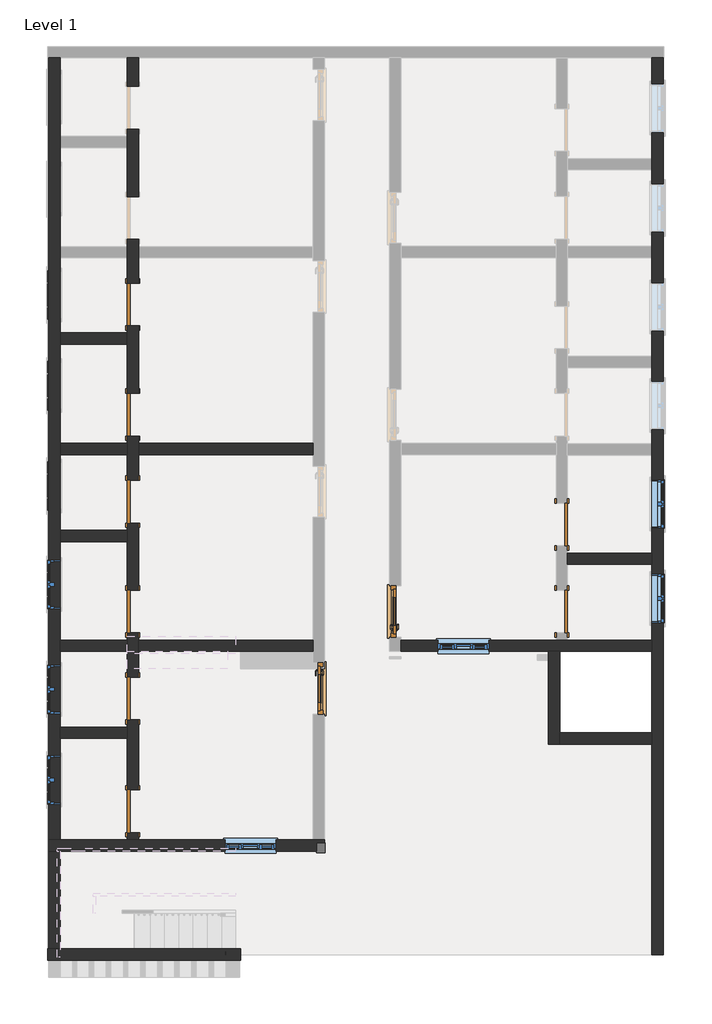
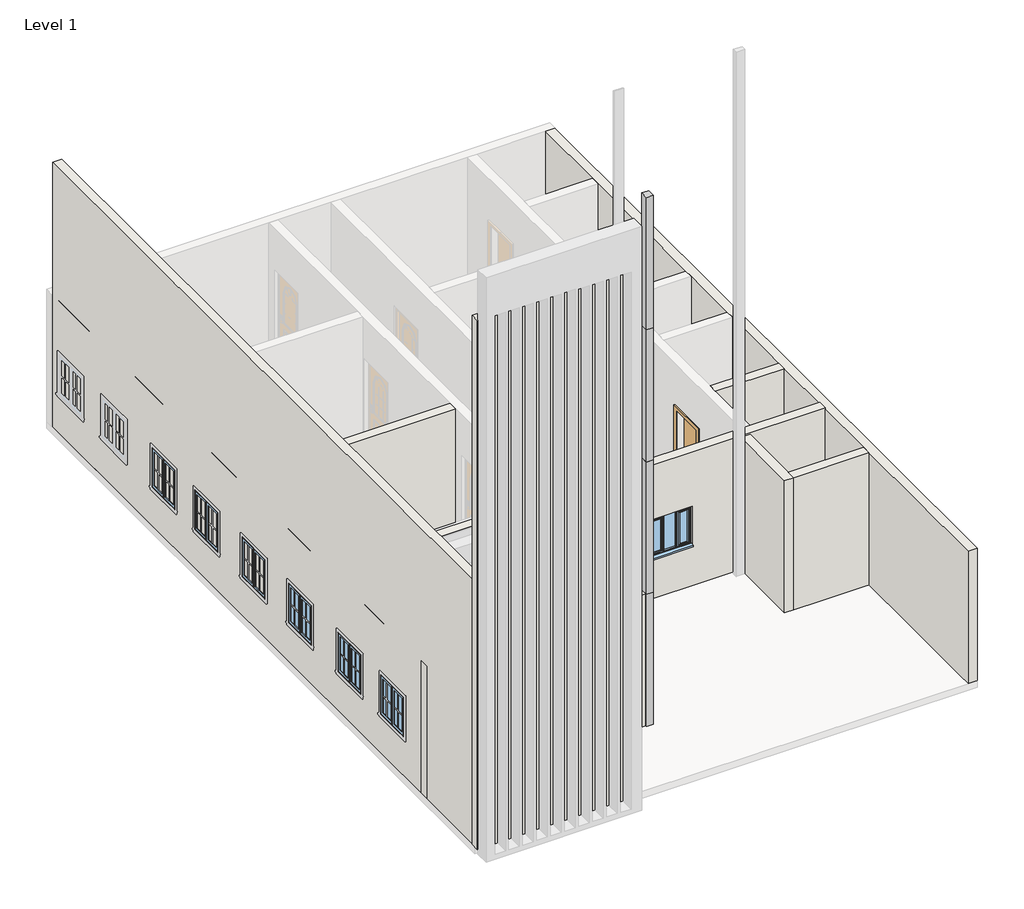
# One storey, part 1 of 4: 17 walls, 10 doors, 10 windows, 1 proxy.
"""IFC4 building model written with IfcOpenShell, lengths in millimetres."""

from ifc_helpers import new_model, si_unit, frame, origin, origin_with_axes, place, context, project, spatial, polyline, outline, extrude, faceted_brep, transform, mapped, element, save
from components import doors_extsgl_w_glazing_bars_arched_910x2110mm_1ab485ba, door_fadea3f2, door_53b1b562, window_c29befe5, windows_tpl_plain_910x910mm_84e79c20

model = new_model("IFC4")

# Units and contexts
model_context = context("Model", 3, world=origin())
ifc_project = project(units=[si_unit("LENGTHUNIT", "METRE", prefix="MILLI")], contexts=[model_context])

# Site, building, storey
site = spatial("IfcSite", under=ifc_project)
building = spatial("IfcBuilding", under=site)
storey = spatial("IfcBuildingStorey", under=building, Name="Level 1", Elevation=0.0)

# Proxy
placement = place(None, origin())
element("IfcBuildingElementProxy", 1, Name="Reveal", ObjectType="Reveal", at=placement, inside=storey, context=model_context, shape_type="SweptSolid", body=[
    extrude(outline(polyline([(-1673.2108866, -6357.2400272), (-1673.2108866, -6174.3600272), (-1520.8108866, -6174.3600272), (-1520.8108866, -6357.2400272), (-1673.2108866, -6357.2400272)])), frame((0.0, 0.0, 9144.0), z_axis=(0.0, 0.0, 1.0), x_axis=(1.0, 0.0, 0.0)), (0.0, 0.0, 1.0), 3048.0),
    extrude(outline(polyline([(-1673.2108866, -6357.2400272), (-1673.2108866, -6174.3600272), (-1520.8108866, -6174.3600272), (-1520.8108866, -6357.2400272), (-1673.2108866, -6357.2400272)])), frame((0.0, 0.0, 6096.0), z_axis=(0.0, 0.0, 1.0), x_axis=(1.0, 0.0, 0.0)), (0.0, 0.0, 1.0), 3048.0),
    extrude(outline(polyline([(-1673.2108866, -6357.2400272), (-1673.2108866, -6174.3600272), (-1520.8108866, -6174.3600272), (-1520.8108866, -6357.2400272), (-1673.2108866, -6357.2400272)])), frame((0.0, 0.0, 3048.0), z_axis=(0.0, 0.0, 1.0), x_axis=(1.0, 0.0, 0.0)), (0.0, 0.0, 1.0), 3048.0),
    extrude(outline(polyline([(-1673.2108866, -6357.2400272), (-1673.2108866, -6174.3600272), (-1520.8108866, -6174.3600272), (-1520.8108866, -6357.2400272), (-1673.2108866, -6357.2400272)])), origin_with_axes(), (0.0, 0.0, 1.0), 3048.0),
])

# Doors
doors_extsgl_w_glazing_bars_arched_910x2110mm_shape = doors_extsgl_w_glazing_bars_arched_910x2110mm_1ab485ba(model_context)
element("IfcDoor", 2, ObjectType="Doors_ExtSgl_w-Glazing_Bars_Arched : 910x2110mm", at=placement, inside=storey, context=model_context, shape_type="MappedRepresentation", body=[
    mapped(doors_extsgl_w_glazing_bars_arched_910x2110mm_shape, transform((-1635.1108866, -3431.1600272, 0.0), x_axis=(0.0, -1.0, 0.0), y_axis=(1.0, 0.0, 0.0), z_axis=(0.0, 0.0, 1.0))),
])
element("IfcDoor", 3, ObjectType="Doors_ExtSgl_w-Glazing_Bars_Arched : 910x2110mm", at=placement, inside=storey, context=model_context, shape_type="MappedRepresentation", body=[
    mapped(doors_extsgl_w_glazing_bars_arched_910x2110mm_shape, transform((-276.2108866, -2059.5600272, 0.0), x_axis=(0.0, 1.0, 0.0), y_axis=(-1.0, 0.0, 0.0), z_axis=(0.0, 0.0, 1.0))),
])
door_shape = door_fadea3f2(model_context)
element("IfcDoor", 4, ObjectType="Single-Flush : 30\" x 80\"", at=placement, inside=storey, context=model_context, shape_type="MappedRepresentation", body=[
    mapped(door_shape, transform((2695.5891134, -510.1600272, 0.0), x_axis=(0.0, -1.0, 0.0), y_axis=(1.0, 0.0, 0.0), z_axis=(0.0, 0.0, 1.0))),
])
element("IfcDoor", 5, ObjectType="Single-Flush : 30\" x 80\"", at=placement, inside=storey, context=model_context, shape_type="MappedRepresentation", body=[
    mapped(door_shape, transform((2695.5891134, -2059.5600272, 0.0), x_axis=(0.0, -1.0, 0.0), y_axis=(1.0, 0.0, 0.0), z_axis=(0.0, 0.0, 1.0))),
])
door_2_shape = door_53b1b562(model_context)
element("IfcDoor", 6, ObjectType="Single-Flush : 30\" x 80\"", at=placement, inside=storey, context=model_context, shape_type="MappedRepresentation", body=[
    mapped(door_2_shape, transform((-4949.8108866, 3407.538843, 0.0), x_axis=(0.0, -1.0, 0.0), y_axis=(1.0, 0.0, 0.0), z_axis=(0.0, 0.0, 1.0))),
])
element("IfcDoor", 7, ObjectType="Single-Flush : 30\" x 80\"", at=placement, inside=storey, context=model_context, shape_type="MappedRepresentation", body=[
    mapped(door_2_shape, transform((-4949.8108866, 1445.6399728, 0.0), x_axis=(0.0, -1.0, 0.0), y_axis=(1.0, 0.0, 0.0), z_axis=(0.0, 0.0, 1.0))),
])
element("IfcDoor", 8, ObjectType="Single-Flush : 30\" x 80\"", at=placement, inside=storey, context=model_context, shape_type="MappedRepresentation", body=[
    mapped(door_2_shape, transform((-4949.8108866, -103.7600272, 0.0), x_axis=(0.0, -1.0, 0.0), y_axis=(1.0, 0.0, 0.0), z_axis=(0.0, 0.0, 1.0))),
])
element("IfcDoor", 9, ObjectType="Single-Flush : 30\" x 80\"", at=placement, inside=storey, context=model_context, shape_type="MappedRepresentation", body=[
    mapped(door_2_shape, transform((-4949.8108866, -2059.5600272, 0.0), x_axis=(0.0, -1.0, 0.0), y_axis=(1.0, 0.0, 0.0), z_axis=(0.0, 0.0, 1.0))),
])
element("IfcDoor", 10, ObjectType="Single-Flush : 30\" x 80\"", at=placement, inside=storey, context=model_context, shape_type="MappedRepresentation", body=[
    mapped(door_2_shape, transform((-4949.8108866, -3608.9600272, 0.0), x_axis=(0.0, -1.0, 0.0), y_axis=(1.0, 0.0, 0.0), z_axis=(0.0, 0.0, 1.0))),
])
element("IfcDoor", 11, ObjectType="Single-Flush : 30\" x 80\"", at=placement, inside=storey, context=model_context, shape_type="MappedRepresentation", body=[
    mapped(door_2_shape, transform((-4949.8108866, -5615.5600272, 0.0), x_axis=(0.0, -1.0, 0.0), y_axis=(1.0, 0.0, 0.0), z_axis=(0.0, 0.0, 1.0))),
])

# Walls
element("IfcWall", 12, ObjectType="4.5\" p", at=placement, inside=storey, context=model_context, shape_type="Brep", body=[
    faceted_brep([(-5051.4108866, -5996.5600272, 2032.0), (-5051.4108866, -5996.5600272, 0.0), (-5051.4108866, -6123.5600272, 0.0), (-5051.4108866, -6123.5600272, 3048.0), (-5051.4108866, -4320.1600272, 3048.0), (-5051.4108866, -4116.9600272, 3048.0), (-5051.4108866, -2770.7600272, 3048.0), (-5051.4108866, -2567.5600272, 3048.0), (-5051.4108866, -814.9600272, 3048.0), (-5051.4108866, -611.7600272, 3048.0), (-5051.4108866, 734.4399728, 3048.0), (-5051.4108866, 937.6399728, 3048.0), (-5051.4108866, 2696.338843, 3048.0), (-5051.4108866, 2899.538843, 3048.0), (-5051.4108866, 4235.1935874, 3048.0), (-5051.4108866, 4438.3935874, 3048.0), (-5051.4108866, 6195.4399728, 3048.0), (-5051.4108866, 6398.6399728, 3048.0), (-5051.4108866, 7795.6399728, 3048.0), (-5051.4108866, 7795.6399728, 0.0), (-5051.4108866, 7287.6399728, 0.0), (-5051.4108866, 7287.6399728, 2032.0), (-5051.4108866, 6525.6399728, 2032.0), (-5051.4108866, 6525.6399728, 0.0), (-5051.4108866, 6398.6399728, 0.0), (-5051.4108866, 6195.4399728, 0.0), (-5051.4108866, 5327.3935874, 0.0), (-5051.4108866, 5327.3935874, 2032.0), (-5051.4108866, 4565.3935874, 2032.0), (-5051.4108866, 4565.3935874, 0.0), (-5051.4108866, 4438.3935874, 0.0), (-5051.4108866, 4235.1935874, 0.0), (-5051.4108866, 3788.538843, 0.0), (-5051.4108866, 3788.538843, 2032.0), (-5051.4108866, 3026.538843, 2032.0), (-5051.4108866, 3026.538843, 0.0), (-5051.4108866, 2899.538843, 0.0), (-5051.4108866, 2696.338843, 0.0), (-5051.4108866, 1826.6399728, 0.0), (-5051.4108866, 1826.6399728, 2032.0), (-5051.4108866, 1064.6399728, 2032.0), (-5051.4108866, 1064.6399728, 0.0), (-5051.4108866, 937.6399728, 0.0), (-5051.4108866, 734.4399728, 0.0), (-5051.4108866, 277.2399728, 0.0), (-5051.4108866, 277.2399728, 2032.0), (-5051.4108866, -484.7600272, 2032.0), (-5051.4108866, -484.7600272, 0.0), (-5051.4108866, -611.7600272, 0.0), (-5051.4108866, -814.9600272, 0.0), (-5051.4108866, -1678.5600272, 0.0), (-5051.4108866, -1678.5600272, 2032.0), (-5051.4108866, -2440.5600272, 2032.0), (-5051.4108866, -2440.5600272, 0.0), (-5051.4108866, -2567.5600272, 0.0), (-5051.4108866, -2770.7600272, 0.0), (-5051.4108866, -3227.9600272, 0.0), (-5051.4108866, -3227.9600272, 2032.0), (-5051.4108866, -3989.9600272, 2032.0), (-5051.4108866, -3989.9600272, 0.0), (-5051.4108866, -4116.9600272, 0.0), (-5051.4108866, -4320.1600272, 0.0), (-5051.4108866, -5234.5600272, 0.0), (-5051.4108866, -5234.5600272, 2032.0), (-4848.2108866, -6123.5600272, 0.0), (-4848.2108866, -5996.5600272, 0.0), (-4848.2108866, -5996.5600272, 2032.0), (-4848.2108866, -5234.5600272, 2032.0), (-4848.2108866, -5234.5600272, 0.0), (-4848.2108866, -3989.9600272, 0.0), (-4848.2108866, -3989.9600272, 2032.0), (-4848.2108866, -3227.9600272, 2032.0), (-4848.2108866, -3227.9600272, 0.0), (-4848.2108866, -2770.7600272, 0.0), (-4848.2108866, -2567.5600272, 0.0), (-4848.2108866, -2440.5600272, 0.0), (-4848.2108866, -2440.5600272, 2032.0), (-4848.2108866, -1678.5600272, 2032.0), (-4848.2108866, -1678.5600272, 0.0), (-4848.2108866, -484.7600272, 0.0), (-4848.2108866, -484.7600272, 2032.0), (-4848.2108866, 277.2399728, 2032.0), (-4848.2108866, 277.2399728, 0.0), (-4848.2108866, 734.4399728, 0.0), (-4848.2108866, 937.6399728, 0.0), (-4848.2108866, 1064.6399728, 0.0), (-4848.2108866, 1064.6399728, 2032.0), (-4848.2108866, 1826.6399728, 2032.0), (-4848.2108866, 1826.6399728, 0.0), (-4848.2108866, 3026.538843, 0.0), (-4848.2108866, 3026.538843, 2032.0), (-4848.2108866, 3788.538843, 2032.0), (-4848.2108866, 3788.538843, 0.0), (-4848.2108866, 4235.1935874, 0.0), (-4848.2108866, 4438.3935874, 0.0), (-4848.2108866, 4565.3935874, 0.0), (-4848.2108866, 4565.3935874, 2032.0), (-4848.2108866, 5327.3935874, 2032.0), (-4848.2108866, 5327.3935874, 0.0), (-4848.2108866, 6525.6399728, 0.0), (-4848.2108866, 6525.6399728, 2032.0), (-4848.2108866, 7287.6399728, 2032.0), (-4848.2108866, 7287.6399728, 0.0), (-4848.2108866, 7795.6399728, 0.0), (-4848.2108866, 7795.6399728, 3048.0), (-4848.2108866, 4438.3935874, 3048.0), (-4848.2108866, 4235.1935874, 3048.0), (-4848.2108866, 937.6399728, 3048.0), (-4848.2108866, 734.4399728, 3048.0), (-4848.2108866, -2567.5600272, 3048.0), (-4848.2108866, -2770.7600272, 3048.0), (-4848.2108866, -6123.5600272, 3048.0)], [[[0, 1, 2, 3, 4, 5, 6, 7, 8, 9, 10, 11, 12, 13, 14, 15, 16, 17, 18, 19, 20, 21, 22, 23, 24, 25, 26, 27, 28, 29, 30, 31, 32, 33, 34, 35, 36, 37, 38, 39, 40, 41, 42, 43, 44, 45, 46, 47, 48, 49, 50, 51, 52, 53, 54, 55, 56, 57, 58, 59, 60, 61, 62, 63]], [[64, 65, 66, 67, 68, 69, 70, 71, 72, 73, 74, 75, 76, 77, 78, 79, 80, 81, 82, 83, 84, 85, 86, 87, 88, 89, 90, 91, 92, 93, 94, 95, 96, 97, 98, 99, 100, 101, 102, 103, 104, 105, 106, 107, 108, 109, 110, 111]], [[20, 19, 103, 102]], [[26, 25, 24, 23, 99, 98]], [[32, 31, 30, 29, 95, 94, 93, 92]], [[38, 37, 36, 35, 89, 88]], [[44, 43, 42, 41, 85, 84, 83, 82]], [[50, 49, 48, 47, 79, 78]], [[56, 55, 54, 53, 75, 74, 73, 72]], [[2, 1, 65, 64]], [[62, 61, 60, 59, 69, 68]], [[18, 17, 16, 15, 14, 13, 12, 11, 10, 9, 8, 7, 6, 5, 4, 3, 111, 110, 109, 108, 107, 106, 105, 104]], [[19, 18, 104, 103]], [[3, 2, 64, 111]], [[100, 99, 23, 22]], [[101, 100, 22, 21]], [[102, 101, 21, 20]], [[96, 95, 29, 28]], [[97, 96, 28, 27]], [[98, 97, 27, 26]], [[90, 89, 35, 34]], [[91, 90, 34, 33]], [[92, 91, 33, 32]], [[86, 85, 41, 40]], [[87, 86, 40, 39]], [[88, 87, 39, 38]], [[80, 79, 47, 46]], [[81, 80, 46, 45]], [[82, 81, 45, 44]], [[76, 75, 53, 52]], [[77, 76, 52, 51]], [[78, 77, 51, 50]], [[70, 69, 59, 58]], [[71, 70, 58, 57]], [[72, 71, 57, 56]], [[66, 65, 1, 0]], [[67, 66, 0, 63]], [[68, 67, 63, 62]]]),
])
element("IfcWall", 13, ObjectType="4.5\" p", at=placement, inside=storey, context=model_context, shape_type="SweptSolid", body=[
    extrude(outline(polyline([(-5051.4108866, 2696.338843), (-6245.2108866, 2696.338843), (-6245.2108866, 2899.538843), (-5051.4108866, 2899.538843), (-5051.4108866, 2696.338843)])), origin_with_axes(), (0.0, 0.0, 1.0), 3048.0),
])
element("IfcWall", 14, ObjectType="4.5\" p", at=placement, inside=storey, context=model_context, shape_type="SweptSolid", body=[
    extrude(outline(polyline([(-5051.4108866, 734.4399728), (-6245.2108866, 734.4399728), (-6245.2108866, 937.6399728), (-5051.4108866, 937.6399728), (-5051.4108866, 734.4399728)])), origin_with_axes(), (0.0, 0.0, 1.0), 3048.0),
])
element("IfcWall", 15, ObjectType="4.5\" p", at=placement, inside=storey, context=model_context, shape_type="SweptSolid", body=[
    extrude(outline(polyline([(-5051.4108866, -814.9600272), (-6245.2108866, -814.9600272), (-6245.2108866, -611.7600272), (-5051.4108866, -611.7600272), (-5051.4108866, -814.9600272)])), origin_with_axes(), (0.0, 0.0, 1.0), 3048.0),
])
element("IfcWall", 16, ObjectType="4.5\" p", at=placement, inside=storey, context=model_context, shape_type="SweptSolid", body=[
    extrude(outline(polyline([(-5051.4108866, -2770.7600272), (-6245.2108866, -2770.7600272), (-6245.2108866, -2567.5600272), (-5051.4108866, -2567.5600272), (-5051.4108866, -2770.7600272)])), origin_with_axes(), (0.0, 0.0, 1.0), 3048.0),
])
element("IfcWall", 17, ObjectType="4.5\" p", at=placement, inside=storey, context=model_context, shape_type="SweptSolid", body=[
    extrude(outline(polyline([(-5051.4108866, -4320.1600272), (-6245.2108866, -4320.1600272), (-6245.2108866, -4116.9600272), (-5051.4108866, -4116.9600272), (-5051.4108866, -4320.1600272)])), origin_with_axes(), (0.0, 0.0, 1.0), 3048.0),
])
element("IfcWall", 18, ObjectType="4.5\" p", at=placement, inside=storey, context=model_context, shape_type="SweptSolid", body=[
    extrude(outline(polyline([(-1736.7108866, 734.4399728), (-4848.2108866, 734.4399728), (-4848.2108866, 937.6399728), (-1736.7108866, 937.6399728), (-1736.7108866, 734.4399728)])), origin_with_axes(), (0.0, 0.0, 1.0), 3048.0),
])
element("IfcWall", 19, ObjectType="4.5\" p", at=placement, inside=storey, context=model_context, shape_type="SweptSolid", body=[
    extrude(outline(polyline([(-1736.7108866, -2770.7600272), (-4848.2108866, -2770.7600272), (-4848.2108866, -2567.5600272), (-1736.7108866, -2567.5600272), (-1736.7108866, -2770.7600272)])), origin_with_axes(), (0.0, 0.0, 1.0), 3048.0),
])
element("IfcWall", 20, ObjectType="4.5\" p", at=placement, inside=storey, context=model_context, shape_type="Brep", body=[
    faceted_brep([(-174.6108866, -2770.7600272, 0.0), (2454.2891134, -2770.7600272, 0.0), (2657.4891134, -2770.7600272, 0.0), (4295.7891134, -2770.7600272, 0.0), (4295.7891134, -2770.7600272, 3088.1226014), (-174.6108866, -2770.7600272, 3088.1226014), (-174.6108866, -2770.7600272, 3048.0), (1397.9891134, -2770.7600272, 1824.4), (1397.9891134, -2770.7600272, 914.4), (487.9891134, -2770.7600272, 914.4), (487.9891134, -2770.7600272, 1824.4), (-174.6108866, -2567.5600272, 0.0), (-174.6108866, -2567.5600272, 3088.1226014), (4295.7891134, -2567.5600272, 3088.1226014), (4295.7891134, -2567.5600272, 0.0), (2797.1891134, -2567.5600272, 0.0), (2593.9891134, -2567.5600272, 0.0), (1397.9891134, -2567.5600272, 1824.4), (487.9891134, -2567.5600272, 1824.4), (487.9891134, -2567.5600272, 914.4), (1397.9891134, -2567.5600272, 914.4)], [[[0, 1, 2, 3, 4, 5, 6], [7, 8, 9, 10]], [[11, 12, 13, 14, 15, 16], [17, 18, 19, 20]], [[3, 2, 1, 0, 11, 16, 15, 14]], [[5, 4, 13, 12]], [[0, 6, 5, 12, 11]], [[4, 3, 14, 13]], [[8, 7, 17, 20]], [[9, 8, 20, 19]], [[10, 9, 19, 18]], [[7, 10, 18, 17]]]),
])
element("IfcWall", 21, ObjectType="4.5\" p", at=placement, inside=storey, context=model_context, shape_type="Brep", body=[
    faceted_brep([(2454.2891134, -2770.7600272, 0.0), (2454.2891134, -4421.7600272, 0.0), (2454.2891134, -4421.7600272, 3048.0), (2454.2891134, -2770.7600272, 3048.0), (2657.4891134, -2770.7600272, 0.0), (2657.4891134, -2770.7600272, 3048.0), (2657.4891134, -4218.5600272, 3048.0), (2657.4891134, -4421.7600272, 3048.0), (2657.4891134, -4421.7600272, 0.0), (2657.4891134, -4218.5600272, 0.0)], [[[0, 1, 2, 3]], [[4, 5, 6, 7, 8, 9]], [[0, 3, 5, 4]], [[2, 1, 8, 7]], [[1, 0, 4, 9, 8]], [[3, 2, 7, 6, 5]]]),
])
element("IfcWall", 22, ObjectType="4.5\" p", at=placement, inside=storey, context=model_context, shape_type="SweptSolid", body=[
    extrude(outline(polyline([(2657.4891134, -4218.5600272), (4295.7891134, -4218.5600272), (4295.7891134, -4421.7600272), (2657.4891134, -4421.7600272), (2657.4891134, -4218.5600272)])), origin_with_axes(), (0.0, 0.0, 1.0), 3048.0),
])
element("IfcWall", 23, ObjectType="4.5\" p", at=placement, inside=storey, context=model_context, shape_type="SweptSolid", body=[
    extrude(outline(polyline([(4295.7891134, -1221.3600272), (2797.1891134, -1221.3600272), (2797.1891134, -1018.1600272), (4295.7891134, -1018.1600272), (4295.7891134, -1221.3600272)])), origin_with_axes(), (0.0, 0.0, 1.0), 3048.0),
])
element("IfcWall", 24, ObjectType="9\" w", at=placement, inside=storey, context=model_context, shape_type="Brep", body=[
    faceted_brep([(-6448.4108866, -6326.7600272, 3048.0), (-6448.4108866, -6326.7600272, 0.0), (-1673.2108866, -6326.7600272, 0.0), (-1673.2108866, -6326.7600272, 3048.0), (-2399.3108866, -6326.7600272, 1824.4), (-2399.3108866, -6326.7600272, 914.4), (-3309.3108866, -6326.7600272, 914.4), (-3309.3108866, -6326.7600272, 1824.4), (-1533.5108866, -6123.5600272, 0.0), (-1736.7108866, -6123.5600272, 0.0), (-4848.2108866, -6123.5600272, 0.0), (-5051.4108866, -6123.5600272, 0.0), (-6245.2108866, -6123.5600272, 0.0), (-6448.4108866, -6123.5600272, 0.0), (-6448.4108866, -6123.5600272, 3048.0), (-6245.2108866, -6123.5600272, 3048.0), (-5051.4108866, -6123.5600272, 3048.0), (-4848.2108866, -6123.5600272, 3048.0), (-1736.7108866, -6123.5600272, 3048.0), (-1533.5108866, -6123.5600272, 3048.0), (-2399.3108866, -6123.5600272, 914.4), (-2399.3108866, -6123.5600272, 1824.4), (-3309.3108866, -6123.5600272, 1824.4), (-3309.3108866, -6123.5600272, 914.4), (-1533.5108866, -6174.3600272, 0.0), (-1673.2108866, -6174.3600272, 0.0), (-1673.2108866, -6174.3600272, 3048.0), (-1533.5108866, -6174.3600272, 3048.0)], [[[0, 1, 2, 3], [4, 5, 6, 7]], [[8, 9, 10, 11, 12, 13, 14, 15, 16, 17, 18, 19], [20, 21, 22, 23]], [[13, 12, 11, 10, 9, 8, 24, 25, 2, 1]], [[19, 18, 17, 16, 15, 14, 0, 3, 26, 27]], [[1, 0, 14, 13]], [[8, 19, 27, 24]], [[5, 4, 21, 20]], [[6, 5, 20, 23]], [[7, 6, 23, 22]], [[4, 7, 22, 21]], [[26, 25, 24, 27]], [[25, 26, 3, 2]]]),
])
element("IfcWall", 25, ObjectType="9\" w", at=placement, inside=storey, context=model_context, shape_type="Brep", body=[
    faceted_brep([(-6448.4108866, 7795.6399728, 0.0), (-6448.4108866, -6123.5600272, 0.0), (-6448.4108866, -6123.5600272, 3048.0), (-6448.4108866, 7795.6399728, 3048.0), (-6448.4108866, 7528.9399728, 1828.8), (-6448.4108866, 6665.3399728, 1828.8), (-6448.4108866, 6665.3399728, 914.4), (-6448.4108866, 7528.9399728, 914.4), (-6448.4108866, 5890.6399728, 1828.8), (-6448.4108866, 5027.0399728, 1828.8), (-6448.4108866, 5027.0399728, 914.4), (-6448.4108866, 5890.6399728, 914.4), (-6448.4108866, 4006.5935874, 1828.8), (-6448.4108866, 3142.9935874, 1828.8), (-6448.4108866, 3142.9935874, 914.4), (-6448.4108866, 4006.5935874, 914.4), (-6448.4108866, 2391.538843, 1828.8), (-6448.4108866, 1527.938843, 1828.8), (-6448.4108866, 1527.938843, 914.4), (-6448.4108866, 2391.538843, 914.4), (-6448.4108866, 607.4399728, 1828.8), (-6448.4108866, -256.1600272, 1828.8), (-6448.4108866, -256.1600272, 914.4), (-6448.4108866, 607.4399728, 914.4), (-6448.4108866, -1145.1600272, 1828.8), (-6448.4108866, -2008.7600272, 1828.8), (-6448.4108866, -2008.7600272, 914.4), (-6448.4108866, -1145.1600272, 914.4), (-6448.4108866, -3012.0600272, 1828.8), (-6448.4108866, -3875.6600272, 1828.8), (-6448.4108866, -3875.6600272, 914.4), (-6448.4108866, -3012.0600272, 914.4), (-6448.4108866, -4624.9600272, 1828.8), (-6448.4108866, -5488.5600272, 1828.8), (-6448.4108866, -5488.5600272, 914.4), (-6448.4108866, -4624.9600272, 914.4), (-6245.2108866, 7795.6399728, 0.0), (-6245.2108866, 7795.6399728, 3048.0), (-6245.2108866, 6398.6399728, 3048.0), (-6245.2108866, 6195.4399728, 3048.0), (-6245.2108866, 4438.3935874, 3048.0), (-6245.2108866, 4235.1935874, 3048.0), (-6245.2108866, 2899.538843, 3048.0), (-6245.2108866, 2696.338843, 3048.0), (-6245.2108866, 937.6399728, 3048.0), (-6245.2108866, 734.4399728, 3048.0), (-6245.2108866, -611.7600272, 3048.0), (-6245.2108866, -814.9600272, 3048.0), (-6245.2108866, -2567.5600272, 3048.0), (-6245.2108866, -2770.7600272, 3048.0), (-6245.2108866, -4116.9600272, 3048.0), (-6245.2108866, -4320.1600272, 3048.0), (-6245.2108866, -6123.5600272, 3048.0), (-6245.2108866, -6123.5600272, 0.0), (-6245.2108866, -4320.1600272, 0.0), (-6245.2108866, -4116.9600272, 0.0), (-6245.2108866, -2770.7600272, 0.0), (-6245.2108866, -2567.5600272, 0.0), (-6245.2108866, -814.9600272, 0.0), (-6245.2108866, -611.7600272, 0.0), (-6245.2108866, 734.4399728, 0.0), (-6245.2108866, 937.6399728, 0.0), (-6245.2108866, 2696.338843, 0.0), (-6245.2108866, 2899.538843, 0.0), (-6245.2108866, 4235.1935874, 0.0), (-6245.2108866, 4438.3935874, 0.0), (-6245.2108866, 6195.4399728, 0.0), (-6245.2108866, 6398.6399728, 0.0), (-6245.2108866, 7528.9399728, 1828.8), (-6245.2108866, 7528.9399728, 914.4), (-6245.2108866, 6665.3399728, 914.4), (-6245.2108866, 6665.3399728, 1828.8), (-6245.2108866, 5890.6399728, 1828.8), (-6245.2108866, 5890.6399728, 914.4), (-6245.2108866, 5027.0399728, 914.4), (-6245.2108866, 5027.0399728, 1828.8), (-6245.2108866, 4006.5935874, 1828.8), (-6245.2108866, 4006.5935874, 914.4), (-6245.2108866, 3142.9935874, 914.4), (-6245.2108866, 3142.9935874, 1828.8), (-6245.2108866, 2391.538843, 1828.8), (-6245.2108866, 2391.538843, 914.4), (-6245.2108866, 1527.938843, 914.4), (-6245.2108866, 1527.938843, 1828.8), (-6245.2108866, 607.4399728, 1828.8), (-6245.2108866, 607.4399728, 914.4), (-6245.2108866, -256.1600272, 914.4), (-6245.2108866, -256.1600272, 1828.8), (-6245.2108866, -1145.1600272, 1828.8), (-6245.2108866, -1145.1600272, 914.4), (-6245.2108866, -2008.7600272, 914.4), (-6245.2108866, -2008.7600272, 1828.8), (-6245.2108866, -3012.0600272, 1828.8), (-6245.2108866, -3012.0600272, 914.4), (-6245.2108866, -3875.6600272, 914.4), (-6245.2108866, -3875.6600272, 1828.8), (-6245.2108866, -4624.9600272, 1828.8), (-6245.2108866, -4624.9600272, 914.4), (-6245.2108866, -5488.5600272, 914.4), (-6245.2108866, -5488.5600272, 1828.8)], [[[0, 1, 2, 3], [4, 5, 6, 7], [8, 9, 10, 11], [12, 13, 14, 15], [16, 17, 18, 19], [20, 21, 22, 23], [24, 25, 26, 27], [28, 29, 30, 31], [32, 33, 34, 35]], [[36, 37, 38, 39, 40, 41, 42, 43, 44, 45, 46, 47, 48, 49, 50, 51, 52, 53, 54, 55, 56, 57, 58, 59, 60, 61, 62, 63, 64, 65, 66, 67], [68, 69, 70, 71], [72, 73, 74, 75], [76, 77, 78, 79], [80, 81, 82, 83], [84, 85, 86, 87], [88, 89, 90, 91], [92, 93, 94, 95], [96, 97, 98, 99]], [[1, 0, 36, 67, 66, 65, 64, 63, 62, 61, 60, 59, 58, 57, 56, 55, 54, 53]], [[3, 2, 52, 51, 50, 49, 48, 47, 46, 45, 44, 43, 42, 41, 40, 39, 38, 37]], [[2, 1, 53, 52]], [[0, 3, 37, 36]], [[69, 68, 4, 7]], [[70, 69, 7, 6]], [[71, 70, 6, 5]], [[68, 71, 5, 4]], [[73, 72, 8, 11]], [[74, 73, 11, 10]], [[75, 74, 10, 9]], [[72, 75, 9, 8]], [[77, 76, 12, 15]], [[78, 77, 15, 14]], [[79, 78, 14, 13]], [[76, 79, 13, 12]], [[81, 80, 16, 19]], [[82, 81, 19, 18]], [[83, 82, 18, 17]], [[80, 83, 17, 16]], [[85, 84, 20, 23]], [[86, 85, 23, 22]], [[87, 86, 22, 21]], [[84, 87, 21, 20]], [[89, 88, 24, 27]], [[90, 89, 27, 26]], [[91, 90, 26, 25]], [[88, 91, 25, 24]], [[93, 92, 28, 31]], [[94, 93, 31, 30]], [[95, 94, 30, 29]], [[92, 95, 29, 28]], [[97, 96, 32, 35]], [[98, 97, 35, 34]], [[99, 98, 34, 33]], [[96, 99, 33, 32]]]),
])
element("IfcWall", 26, ObjectType="9\" w", at=placement, inside=storey, context=model_context, shape_type="Brep", body=[
    faceted_brep([(4295.7891134, 7795.6399728, 0.0), (4295.7891134, 6004.9399728, 0.0), (4295.7891134, 5801.7399728, 0.0), (4295.7891134, 4442.8399728, 0.0), (4295.7891134, 4239.6399728, 0.0), (4295.7891134, 2487.0399728, 0.0), (4295.7891134, 2283.8399728, 0.0), (4295.7891134, 924.9399728, 0.0), (4295.7891134, 721.7399728, 0.0), (4295.7891134, -1018.1600272, 0.0), (4295.7891134, -1221.3600272, 0.0), (4295.7891134, -2567.5600272, 0.0), (4295.7891134, -2770.7600272, 0.0), (4295.7891134, -4218.5600272, 0.0), (4295.7891134, -4421.7600272, 0.0), (4295.7891134, -8168.2600272, 0.0), (4295.7891134, -8168.2600272, 3048.0), (4295.7891134, -4421.7600272, 3048.0), (4295.7891134, -4218.5600272, 3048.0), (4295.7891134, -1221.3600272, 3048.0), (4295.7891134, -1018.1600272, 3048.0), (4295.7891134, 721.7399728, 3048.0), (4295.7891134, 924.9399728, 3048.0), (4295.7891134, 2283.8399728, 3048.0), (4295.7891134, 2487.0399728, 3048.0), (4295.7891134, 4239.6399728, 3048.0), (4295.7891134, 4442.8399728, 3048.0), (4295.7891134, 5801.7399728, 3048.0), (4295.7891134, 6004.9399728, 3048.0), (4295.7891134, 7795.6399728, 3048.0), (4295.7891134, -2262.7600272, 1828.8), (4295.7891134, -2262.7600272, 914.4), (4295.7891134, -1399.1600272, 914.4), (4295.7891134, -1399.1600272, 1828.8), (4295.7891134, -580.0100272, 1828.8), (4295.7891134, -580.0100272, 914.4), (4295.7891134, 283.5899728, 914.4), (4295.7891134, 283.5899728, 1828.8), (4295.7891134, 1172.5899728, 1828.8), (4295.7891134, 1172.5899728, 914.4), (4295.7891134, 2036.1899728, 914.4), (4295.7891134, 2036.1899728, 1828.8), (4295.7891134, 2931.5399728, 1828.8), (4295.7891134, 2931.5399728, 914.4), (4295.7891134, 3795.1399728, 914.4), (4295.7891134, 3795.1399728, 1828.8), (4295.7891134, 4690.4899728, 1828.8), (4295.7891134, 4690.4899728, 914.4), (4295.7891134, 5554.0899728, 914.4), (4295.7891134, 5554.0899728, 1828.8), (4295.7891134, 6468.4899728, 1828.8), (4295.7891134, 6468.4899728, 914.4), (4295.7891134, 7332.0899728, 914.4), (4295.7891134, 7332.0899728, 1828.8), (4498.9891134, 7795.6399728, 0.0), (4498.9891134, 7795.6399728, 3048.0), (4498.9891134, -8168.2600272, 3048.0), (4498.9891134, -8168.2600272, 0.0), (4498.9891134, -2262.7600272, 1828.8), (4498.9891134, -1399.1600272, 1828.8), (4498.9891134, -1399.1600272, 914.4), (4498.9891134, -2262.7600272, 914.4), (4498.9891134, -580.0100272, 1828.8), (4498.9891134, 283.5899728, 1828.8), (4498.9891134, 283.5899728, 914.4), (4498.9891134, -580.0100272, 914.4), (4498.9891134, 1172.5899728, 1828.8), (4498.9891134, 2036.1899728, 1828.8), (4498.9891134, 2036.1899728, 914.4), (4498.9891134, 1172.5899728, 914.4), (4498.9891134, 2931.5399728, 1828.8), (4498.9891134, 3795.1399728, 1828.8), (4498.9891134, 3795.1399728, 914.4), (4498.9891134, 2931.5399728, 914.4), (4498.9891134, 4690.4899728, 1828.8), (4498.9891134, 5554.0899728, 1828.8), (4498.9891134, 5554.0899728, 914.4), (4498.9891134, 4690.4899728, 914.4), (4498.9891134, 6468.4899728, 1828.8), (4498.9891134, 7332.0899728, 1828.8), (4498.9891134, 7332.0899728, 914.4), (4498.9891134, 6468.4899728, 914.4)], [[[0, 1, 2, 3, 4, 5, 6, 7, 8, 9, 10, 11, 12, 13, 14, 15, 16, 17, 18, 19, 20, 21, 22, 23, 24, 25, 26, 27, 28, 29], [30, 31, 32, 33], [34, 35, 36, 37], [38, 39, 40, 41], [42, 43, 44, 45], [46, 47, 48, 49], [50, 51, 52, 53]], [[54, 55, 56, 57], [58, 59, 60, 61], [62, 63, 64, 65], [66, 67, 68, 69], [70, 71, 72, 73], [74, 75, 76, 77], [78, 79, 80, 81]], [[15, 14, 13, 12, 11, 10, 9, 8, 7, 6, 5, 4, 3, 2, 1, 0, 54, 57]], [[16, 15, 57, 56]], [[29, 28, 27, 26, 25, 24, 23, 22, 21, 20, 19, 18, 17, 16, 56, 55]], [[0, 29, 55, 54]], [[31, 30, 58, 61]], [[32, 31, 61, 60]], [[33, 32, 60, 59]], [[30, 33, 59, 58]], [[35, 34, 62, 65]], [[36, 35, 65, 64]], [[37, 36, 64, 63]], [[34, 37, 63, 62]], [[39, 38, 66, 69]], [[40, 39, 69, 68]], [[41, 40, 68, 67]], [[38, 41, 67, 66]], [[43, 42, 70, 73]], [[44, 43, 73, 72]], [[45, 44, 72, 71]], [[42, 45, 71, 70]], [[47, 46, 74, 77]], [[48, 47, 77, 76]], [[49, 48, 76, 75]], [[46, 49, 75, 74]], [[51, 50, 78, 81]], [[52, 51, 81, 80]], [[53, 52, 80, 79]], [[50, 53, 79, 78]]]),
])
element("IfcWall", 27, ObjectType="9\" w", at=placement, inside=storey, context=model_context, shape_type="Brep", body=[
    faceted_brep([(-6461.1108866, -8269.8600272, 0.0), (-3032.1108866, -8269.8600272, 0.0), (-3032.1108866, -8269.8600272, 12192.0), (-6461.1108866, -8269.8600272, 12192.0), (-6461.1108866, -8066.6600272, 0.0), (-6461.1108866, -8066.6600272, 12192.0), (-3032.1108866, -8066.6600272, 12192.0), (-3032.1108866, -8066.6600272, 0.0), (-6245.2108866, -8066.6600272, 0.0), (-6448.4108866, -8066.6600272, 0.0)], [[[0, 1, 2, 3]], [[4, 5, 6, 7, 8, 9]], [[1, 0, 4, 9, 8, 7]], [[2, 1, 7, 6]], [[3, 2, 6, 5]], [[0, 3, 5, 4]]]),
])
element("IfcWall", 28, ObjectType="9\" w", at=placement, inside=storey, context=model_context, shape_type="SweptSolid", body=[
    extrude(outline(polyline([(-6245.2108866, 7795.6399728), (-6245.2108866, -8066.6600272), (-6448.4108866, -8066.6600272), (-6448.4108866, 7795.6399728), (-6245.2108866, 7795.6399728)])), origin_with_axes(), (0.0, 0.0, 1.0), 6096.0),
])

# Windows
window_shape = window_c29befe5(model_context)
element("IfcWindow", 29, ObjectType="Window-Casement-Double : 34\" x 36\"", at=placement, inside=storey, context=model_context, shape_type="MappedRepresentation", body=[
    mapped(window_shape, transform((-6346.8108866, 3574.7935874, 0.0), x_axis=(0.0, 1.0, 0.0), y_axis=(-1.0, 0.0, 0.0), z_axis=(0.0, 0.0, 1.0))),
])
element("IfcWindow", 30, ObjectType="Window-Casement-Double : 34\" x 36\"", at=placement, inside=storey, context=model_context, shape_type="MappedRepresentation", body=[
    mapped(window_shape, transform((-6346.8108866, 1959.738843, 0.0), x_axis=(0.0, 1.0, 0.0), y_axis=(-1.0, 0.0, 0.0), z_axis=(0.0, 0.0, 1.0))),
])
element("IfcWindow", 31, ObjectType="Window-Casement-Double : 34\" x 36\"", at=placement, inside=storey, context=model_context, shape_type="MappedRepresentation", body=[
    mapped(window_shape, transform((-6346.8108866, 175.6399728, 0.0), x_axis=(0.0, 1.0, 0.0), y_axis=(-1.0, 0.0, 0.0), z_axis=(0.0, 0.0, 1.0))),
])
element("IfcWindow", 32, ObjectType="Window-Casement-Double : 34\" x 36\"", at=placement, inside=storey, context=model_context, shape_type="MappedRepresentation", body=[
    mapped(window_shape, transform((-6346.8108866, -1576.9600272, 0.0), x_axis=(0.0, 1.0, 0.0), y_axis=(-1.0, 0.0, 0.0), z_axis=(0.0, 0.0, 1.0))),
])
element("IfcWindow", 33, ObjectType="Window-Casement-Double : 34\" x 36\"", at=placement, inside=storey, context=model_context, shape_type="MappedRepresentation", body=[
    mapped(window_shape, transform((-6346.8108866, -3443.8600272, 0.0), x_axis=(0.0, 1.0, 0.0), y_axis=(-1.0, 0.0, 0.0), z_axis=(0.0, 0.0, 1.0))),
])
element("IfcWindow", 34, ObjectType="Window-Casement-Double : 34\" x 36\"", at=placement, inside=storey, context=model_context, shape_type="MappedRepresentation", body=[
    mapped(window_shape, transform((-6346.8108866, -5056.7600272, 0.0), x_axis=(0.0, 1.0, 0.0), y_axis=(-1.0, 0.0, 0.0), z_axis=(0.0, 0.0, 1.0))),
])
element("IfcWindow", 35, ObjectType="Window-Casement-Double : 34\" x 36\"", at=placement, inside=storey, context=model_context, shape_type="MappedRepresentation", body=[
    mapped(window_shape, transform((4397.3891134, -1830.9600272, 0.0), x_axis=(0.0, -1.0, 0.0), y_axis=(1.0, 0.0, 0.0), z_axis=(0.0, 0.0, 1.0))),
])
element("IfcWindow", 36, ObjectType="Window-Casement-Double : 34\" x 36\"", at=placement, inside=storey, context=model_context, shape_type="MappedRepresentation", body=[
    mapped(window_shape, transform((4397.3891134, -148.2100272, 0.0), x_axis=(0.0, -1.0, 0.0), y_axis=(1.0, 0.0, 0.0), z_axis=(0.0, 0.0, 1.0))),
])
windows_tpl_plain_910x910mm_shape = windows_tpl_plain_910x910mm_84e79c20(model_context)
element("IfcWindow", 37, ObjectType="Windows_Tpl_Plain : 910x910mm", at=placement, inside=storey, context=model_context, shape_type="MappedRepresentation", body=[
    mapped(windows_tpl_plain_910x910mm_shape, transform((516.3224468, -2660.7034594, -285.6), x_axis=(-1.0, 0.0, 0.0), y_axis=(0.0, -1.0, 0.0), z_axis=(0.0, 0.0, 1.0))),
])
element("IfcWindow", 38, ObjectType="Windows_Tpl_Plain : 910x910mm", at=placement, inside=storey, context=model_context, shape_type="MappedRepresentation", body=[
    mapped(windows_tpl_plain_910x910mm_shape, transform((-3280.9775532, -6216.7034594, -285.6), x_axis=(-1.0, 0.0, 0.0), y_axis=(0.0, -1.0, 0.0), z_axis=(0.0, 0.0, 1.0))),
])

save(model, "model.ifc")

# Revit data of these elements
# Type "Doors_ExtSgl_w-Glazing_Bars_Arched : 910x2110mm"
#   Type Mark = "19"
#   Type Comments = "External Single"
#   Operation = "SingleSwingRight"
#   Construction Type Id = "SGL"
#   Keynote = "L20"
#   Analytic Construction = "Large single-glazed windows"
#   Wrap Layers (Int) from Ext = 0' - 6.98819"
#   Wrap Layers (Ext) from Ext = 0' - 4.03543"
#   Visual Light Transmittance = 0.9
#   Thickness = 0' - 1.73228"
#   Solar Heat Gain Coefficient = 0.86
#   Rough Width = 2' - 11.82677"
#   Rough Height = 6' - 11.07087"
#   O/A Frame Width = 0' - 2.51969"
#   Heat Transfer Coefficient (U) = 0.979472 BTU/(h·ft²·°F)
#   Handle Z Distance = 3' - 5.33858"
#   Glazing Thickness = 0' - 0.94488"
#   FrameWidth = 0' - 1.65354"
#   FrameOffset - External = 0' - 0.98425"
#   FrameDepth = 0' - 3.50394"
#   Door Panel Width = 2' - 7.77165"
#   Door Panel Thickness = 0' - 1.73228"
#   Door Panel Height = 6' - 6.74016"
#   DONT CHANGE - Half Glazed Width = 0' - 9.98031"
#   DONT CHANGE - Glazed Width = 1' - 7.96063"
#   Cill Thickness = 0' - 2.14567"
#   Cill Projection = 0' - 1.1811"
#   Handle X Distance = 0' - 2.95276"
#   Height = 6' - 11.07087"
#   Structural Tolerance = 0' - 0.25591"
#   Tolerance = 0' - 0.11811"
#   Undercut = 0' - 0.15748"
#   Width = 2' - 11.82677"
#   Cill Extension = 0' - 0.98425"
#   Cavity Closer Width = 0' - 1.9685"
#   Cavity Closer Offset from Ext = 0' - 4.03543"
#   Cavity Closer Depth = 0' - 3.34646"
#   Vis - Ironmongery = yes
#   Vis - Glazing Bars = yes
#   Vis - Cavity Closers = yes
#   Define Thermal Properties by = 1
#   Function = 1
#   Material Glass = Door - Glazing
#   Material Glazing Bar = Door - Panel
#   Material Door = Door - Panel
#   Material Frame = Door - Frame/Mullion
#   Material Ironmongery = Door - Handle
#   Wall Closure = (empty or 0)
# Type "Single-Flush : 30\" x 80\""
#   Type Mark = "5"
#   Construction Type Id = "MDOOR"
#   Assembly Code = "C1020"
#   Analytic Construction = "Metal"
#   Thickness = 0' - 2"
#   Heat Transfer Coefficient (U) = 0.651978 BTU/(h·ft²·°F)
#   Height = 6' - 8"
#   Trim Projection Ext = 0' - 1"
#   Trim Projection Int = 0' - 1"
#   Trim Width = 0' - 3"
#   Width = 2' - 6"
#   Define Thermal Properties by = 1
#   Define Thermal Properties by = 1
#   Door Material = Door - Panel
#   Frame Material = Door - Frame
#   Visual Light Transmittance = 0
#   Solar Heat Gain Coefficient = 0
#   Function = (empty or 0)
#   Wall Closure = (empty or 0)
# Type "4.5\" p"
#   Assembly Code = "B2010"
#   Layers, outside or top first: 0' - 8" no material (function 1)
# Type "9\" w"
#   Assembly Code = "B2010"
#   Layers, outside or top first: 0' - 8" no material (function 1)
# Type "Window-Casement-Double : 34\" x 36\""
#   Type Mark = "14"
#   Fire Rating = "0.5h"
#   Assembly Code = "B2020100"
#   Analytic Construction = "Double glazing - domestic"
#   Frame Extension [instance default] = 0' - 0 1/4"
#   Window Inset [instance default] = 0' - 0"
#   Wall Thickness [instance default] = 0' - 6"
#   Interior Wall Closure [instance default] = 0' - 2 1/4"
#   Half Width = 1' - 5"
#   Visual Light Transmittance = 0.81
#   Thermal Resistance (R) = 1.8146 (h·ft²·°F)/BTU
#   Solar Heat Gain Coefficient = 0.76
#   Rough Width = 2' - 10 1/2"
#   Rough Height = 3' - 0 1/2"
#   Height = 3' - 0"
#   Heat Transfer Coefficient (U) = 0.5511 BTU/(h·ft²·°F)
#   Exterior Wall Closure [instance default] = 0' - 1 1/4"
#   Extension Jamb [instance default] = 0' - 2 1/4"
#   Default Sill Height = 3' - 0"
#   Width = 2' - 10"
#   Define Thermal Properties by = 0
#   Muntin Visibility = yes
#   Interior Trim Visibility [instance default] = yes
#   Exterior Trim Visibility [instance default] = yes
#   Extension Jamb Visibility [instance default] = yes
#   Interior Trim Material = Wood - Stained
#   Muntin Pattern = Muntin Pattern_2x2 : Muntin Pattern_2x2
#   Interior Trim = Trim-Window-Interior-Flat : Picture Frame
#   Interior Frame Material = Wood - Stained
#   Glass Panel Material = Glass
#   Exterior Trim Material = Clad - White
#   Exterior Trim = Trim-Window-Exterior-Flat : with Sill
#   Exterior Frame Material = Clad - White
#   Wall Closure = (empty or 0)
# Type "Windows_Tpl_Plain : 910x910mm"
#   Type Mark = "18"
#   Operation = "TriplePanelVertical"
#   Construction Type Id = "GSP4R"
#   Manufacturer = "Revit"
#   Keynote = "L10"
#   Analytic Construction = "1/8 in Pilkington single glazing"
#   Wrap Layers (Ext) from Ext = 0' - 4.03543"
#   Wrap Layers (Int) from Ext = 0' - 6.98819"
#   Window Board Projection = 0' - 0.98425"
#   Window Board Extension = 0' - 0.98425"
#   Visual Light Transmittance = 0.9
#   Solar Heat Gain Coefficient = 0.78
#   Rough Width = 2' - 11.82677"
#   Rough Height = 2' - 11.82677"
#   Height = 2' - 11.82677"
#   Width = 2' - 11.82677"
#   Heat Transfer Coefficient (U) = 0.6496 BTU/(h·ft²·°F)
#   Glazing Thickness = 0' - 0.94488"
#   FrameOffset - External = 0' - 1.9685"
#   Frame Depth = 0' - 2.55906"
#   Default Head Height = 6' - 11.07087"
#   Cill Depth = 0' - 3.44488"
#   Cavity Closer Width = 0' - 1.9685"
#   Cavity Closer Offset from Ext = 0' - 4.03543"
#   Cavity Closer Depth = 0' - 3.34646"
#   Vis - Cavity Closers = yes
#   Define Thermal Properties by = 1
#   Material Trim = Window Frame
#   Material Glass = Glass
#   Material Frame = Window Frame
#   Wall Closure = (empty or 0)
# Elements 2, 3 (IfcDoor, "Doors_ExtSgl_w-Glazing_Bars_Arched : 910x2110mm")
#   Phase Created = New Construction
#   Materials on its faces: "Door - Panel", "Door - Handle", "Door - Frame/Mullion", "Door - Glazing"
# Elements 4, 5, 6, 7, 8, 9, 10, 11 (IfcDoor, "Single-Flush : 30\" x 80\"")
#   Phase Created = New Construction
#   Materials on its faces: "Door - Frame", "Door - Panel"
# Elements 12, 13, 14, 15, 16, 17, 18, 19, 23 (IfcWall, "4.5\" p")
#   Top Offset = 0' - 0"
#   Base Offset = 0' - 0"
#   wall height = 10' - 0"
#   Phase Created = New Construction
#   Base Constraint = Level 1
#   Top Constraint = Level 2
#   Materials on its faces: "Default Wall"
# Element 20 (IfcWall, "4.5\" p")
#   Top Offset = 0' - 1.57963"
#   Base Offset = 0' - 0"
#   wall height = 10' - 1.57963"
#   Phase Created = New Construction
#   Base Constraint = Level 1
#   Top Constraint = Level 2
#   Materials on its faces: "Default Wall", "Window Frame", "Cherry"
# Elements 21, 22 (IfcWall, "4.5\" p")
#   Top Offset = 0' - 0"
#   Base Offset = 0' - 0"
#   wall height = 10' - 0"
#   Phase Created = New Construction
#   Base Constraint = Level 1
#   Top Constraint = Level 2
#   Materials on its faces: "Default Wall", "Doors - Glazing Bars"
# Element 24 (IfcWall, "9\" w")
#   Top Offset = 0' - 0"
#   Base Offset = 0' - 0"
#   wall height = 10' - 0"
#   Phase Created = New Construction
#   Base Constraint = Level 1
#   Top Constraint = Level 2
#   Materials on its faces: "Default Wall", "Wood - Stained", "Brick, Common"
# Element 25 (IfcWall, "9\" w")
#   Top Offset = 0' - 0"
#   Base Offset = 0' - 0"
#   wall height = 10' - 0"
#   Phase Created = New Construction
#   Base Constraint = Level 1
#   Top Constraint = Level 2
#   Materials on its faces: "Default Wall"
# Element 26 (IfcWall, "9\" w")
#   Top Offset = 0' - 0"
#   Base Offset = 0' - 0"
#   wall height = 10' - 0"
#   Phase Created = New Construction
#   Base Constraint = Level 1
#   Top Constraint = Level 2
#   Materials on its faces: "Default Wall", "Wood - Stained", "Earth"
# Element 27 (IfcWall, "9\" w")
#   Top Offset = 0' - 0"
#   Base Offset = 0' - 0"
#   Unconnected Height = 40' - 0"
#   wall height = 40' - 0"
#   Phase Created = New Construction
#   Base Constraint = Level 1
#   Materials on its faces: "Default Wall", "Doors - Glazing Bars", "Wood - Stained"
# Element 28 (IfcWall, "9\" w")
#   Top Offset = 0' - 0"
#   Base Offset = 0' - 0"
#   Unconnected Height = 20' - 0"
#   wall height = 20' - 0"
#   Phase Created = New Construction
#   Base Constraint = Level 1
#   Materials on its faces: "Default Wall", "Wood - Stained"
# Element 29 (IfcWindow, "Window-Casement-Double : 34\" x 36\"")
#   Mark = "3"
#   Window Inset = 0' - 0"
#   Interior Wall Closure = 0' - 2 1/4"
#   Frame Extension = 0' - 0 1/4"
#   Exterior Wall Closure = 0' - 1 1/4"
#   Interior Trim Visibility = yes
#   Exterior Trim Visibility = yes
#   Phase Created = New Construction
#   Materials on its faces: "Wood - Stained", "Glass", "Clad - White"
# Element 30 (IfcWindow, "Window-Casement-Double : 34\" x 36\"")
#   Mark = "4"
#   Window Inset = 0' - 0"
#   Interior Wall Closure = 0' - 2 1/4"
#   Frame Extension = 0' - 0 1/4"
#   Exterior Wall Closure = 0' - 1 1/4"
#   Interior Trim Visibility = yes
#   Exterior Trim Visibility = yes
#   Phase Created = New Construction
#   Materials on its faces: "Wood - Stained", "Glass", "Clad - White"
# Element 31 (IfcWindow, "Window-Casement-Double : 34\" x 36\"")
#   Mark = "5"
#   Window Inset = 0' - 0"
#   Interior Wall Closure = 0' - 2 1/4"
#   Frame Extension = 0' - 0 1/4"
#   Exterior Wall Closure = 0' - 1 1/4"
#   Interior Trim Visibility = yes
#   Exterior Trim Visibility = yes
#   Phase Created = New Construction
#   Materials on its faces: "Wood - Stained", "Glass", "Clad - White"
# Element 32 (IfcWindow, "Window-Casement-Double : 34\" x 36\"")
#   Mark = "6"
#   Window Inset = 0' - 0"
#   Interior Wall Closure = 0' - 2 1/4"
#   Frame Extension = 0' - 0 1/4"
#   Exterior Wall Closure = 0' - 1 1/4"
#   Interior Trim Visibility = yes
#   Exterior Trim Visibility = yes
#   Phase Created = New Construction
#   Materials on its faces: "Wood - Stained", "Glass", "Clad - White"
# Element 33 (IfcWindow, "Window-Casement-Double : 34\" x 36\"")
#   Mark = "7"
#   Window Inset = 0' - 0"
#   Interior Wall Closure = 0' - 2 1/4"
#   Frame Extension = 0' - 0 1/4"
#   Exterior Wall Closure = 0' - 1 1/4"
#   Interior Trim Visibility = yes
#   Exterior Trim Visibility = yes
#   Phase Created = New Construction
#   Materials on its faces: "Wood - Stained", "Glass", "Clad - White"
# Element 34 (IfcWindow, "Window-Casement-Double : 34\" x 36\"")
#   Mark = "8"
#   Window Inset = 0' - 0"
#   Interior Wall Closure = 0' - 2 1/4"
#   Frame Extension = 0' - 0 1/4"
#   Exterior Wall Closure = 0' - 1 1/4"
#   Interior Trim Visibility = yes
#   Exterior Trim Visibility = yes
#   Phase Created = New Construction
#   Materials on its faces: "Wood - Stained", "Glass", "Clad - White"
# Element 35 (IfcWindow, "Window-Casement-Double : 34\" x 36\"")
#   Mark = "9"
#   Window Inset = 0' - 0"
#   Interior Wall Closure = 0' - 2 1/4"
#   Frame Extension = 0' - 0 1/4"
#   Exterior Wall Closure = 0' - 1 1/4"
#   Interior Trim Visibility = yes
#   Exterior Trim Visibility = yes
#   Phase Created = New Construction
#   Materials on its faces: "Wood - Stained", "Glass", "Clad - White"
# Element 36 (IfcWindow, "Window-Casement-Double : 34\" x 36\"")
#   Mark = "10"
#   Window Inset = 0' - 0"
#   Interior Wall Closure = 0' - 2 1/4"
#   Frame Extension = 0' - 0 1/4"
#   Exterior Wall Closure = 0' - 1 1/4"
#   Interior Trim Visibility = yes
#   Exterior Trim Visibility = yes
#   Phase Created = New Construction
#   Materials on its faces: "Wood - Stained", "Glass", "Clad - White"
# Element 37 (IfcWindow, "Windows_Tpl_Plain : 910x910mm")
#   Mark = "15"
#   Phase Created = New Construction
#   Materials on its faces: "Window Frame", "Glass"
# Element 38 (IfcWindow, "Windows_Tpl_Plain : 910x910mm")
#   Mark = "16"
#   Phase Created = New Construction
#   Materials on its faces: "Window Frame", "Glass"
# Materials
#   "Door - Glazing": colour RGB 0 0 255, transparency 0.75
#   "Door - Panel": class "Wood", colour RGB 210 159 95, transparency 0, Cost = 0
#   "Door - Frame/Mullion": class "Wood", colour RGB 212 179 113, transparency 0
#   "Door - Handle": colour RGB 247 247 247, transparency 0
#   "Door - Frame": colour RGB 118 70 51, transparency 0, Cost = 0
#   "Wood - Stained": class "Wood", colour RGB 224 178 126, transparency 0, Cost = 0
#   "Glass": class "Glass", colour RGB 0 128 192, transparency 0.75, Description = "Soda Lime Glass", Cost = 0
#   "Clad - White": class "Wood", colour RGB 242 242 238, transparency 0, Cost = 0
#   "Window Frame": colour RGB 249 249 249, transparency 0
#   "Default Wall": colour RGB 128 128 128, transparency 0, Cost = 0
#   "Cherry": class "Wood", colour RGB 226 177 128, transparency 0, Description = "Prunus Serotina", Cost = 0
#   "Doors - Glazing Bars": colour RGB 158 107 65, transparency 0
#   "Brick, Common": class "Masonry", colour RGB 170 98 104, transparency 0, Description = "Common brick", Cost = 0
#   "Earth": class "Generic", colour RGB 97 75 62, transparency 0, Description = "Soil", Cost = 0
